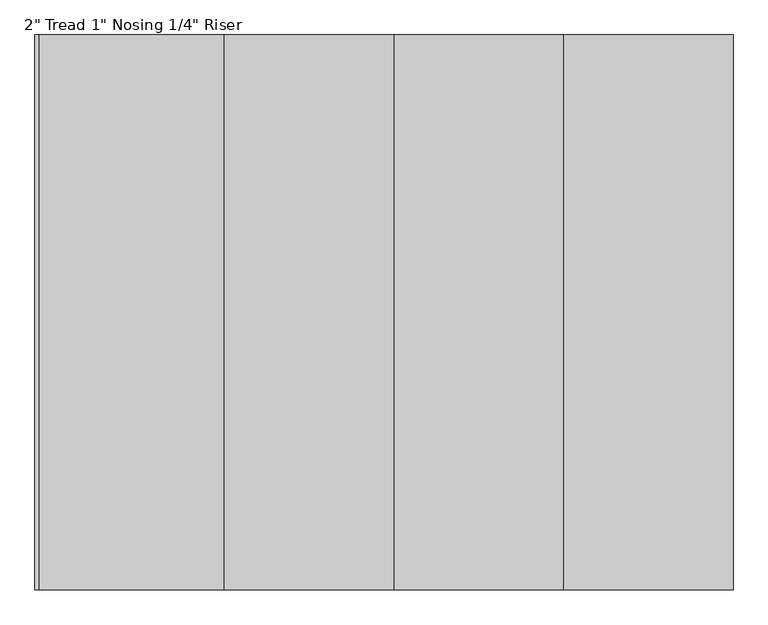
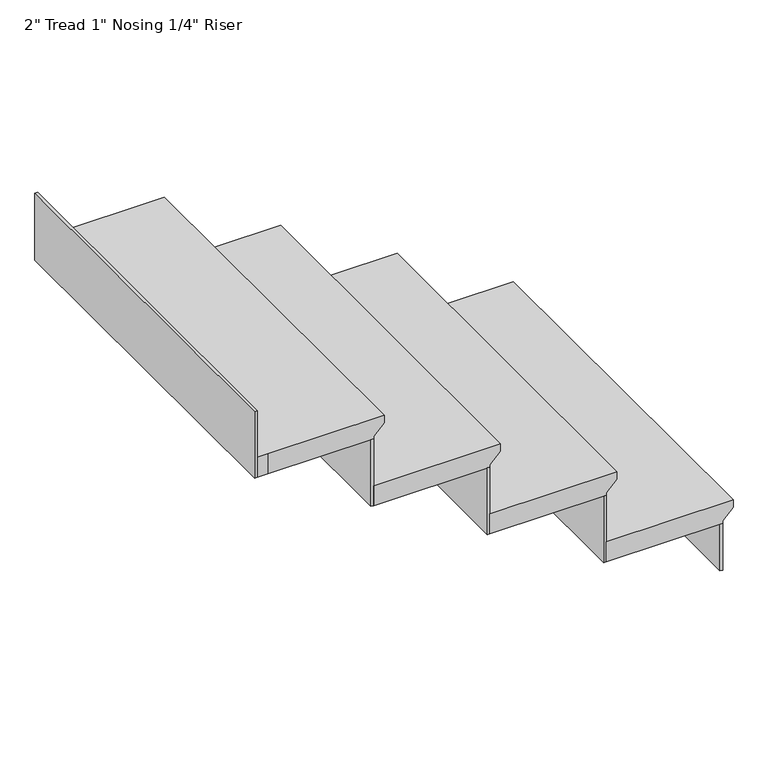
"""IFC4 building model written with IfcOpenShell, lengths in millimetres: stair flight geometry."""

from ifc_helpers import new_model, si_unit, origin, place, context, project, spatial, faceted_brep, source, transform, mapped, element, save


def stair_flight_f80b6bc8(model_context):
    return source(origin(), model_context, "Body", "Brep", [
        faceted_brep([(-9079.7156858, 1045.1115003, 3503.0833333), (-9079.7156858, 1045.1115003, 3522.1333333), (-9079.7156858, 130.7115003, 3522.1333333), (-9079.7156858, 130.7115003, 3503.0833333), (-9105.1156858, 1045.1115003, 3477.6833333), (-9105.1156858, 130.7115003, 3477.6833333), (-9384.5156858, 1045.1115003, 3522.1333333), (-9384.5156858, 130.7115003, 3522.1333333), (-9105.1156858, 130.7115003, 3471.3333333), (-9384.5156858, 130.7115003, 3471.3333333), (-9384.5156858, 1045.1115003, 3471.3333333), (-9105.1156858, 1045.1115003, 3471.3333333)], [[[0, 1, 2, 3]], [[4, 0, 3, 5]], [[2, 1, 6, 7]], [[8, 9, 10, 11]], [[2, 7, 9, 8, 5, 3]], [[8, 11, 4, 5]], [[6, 1, 0, 4, 11, 10]], [[7, 6, 10, 9]]]),
        faceted_brep([(-9105.1156858, 1045.1115003, 3471.3333333), (-9105.1156858, 1045.1115003, 3352.8), (-9111.4656858, 1045.1115003, 3352.8), (-9111.4656858, 1045.1115003, 3471.3333333), (-9105.1156858, 130.7115003, 3471.3333333), (-9111.4656858, 130.7115003, 3471.3333333), (-9111.4656858, 130.7115003, 3352.8), (-9105.1156858, 130.7115003, 3352.8)], [[[0, 1, 2, 3]], [[4, 5, 6, 7]], [[1, 0, 4, 7]], [[2, 1, 7, 6]], [[3, 2, 6, 5]], [[0, 3, 5, 4]]]),
        faceted_brep([(-9384.5156858, 1045.1115003, 3640.6666667), (-9384.5156858, 1045.1115003, 3471.3333333), (-9390.8656858, 1045.1115003, 3471.3333333), (-9390.8656858, 1045.1115003, 3640.6666667), (-9384.5156858, 130.7115003, 3640.6666667), (-9390.8656858, 130.7115003, 3640.6666667), (-9390.8656858, 130.7115003, 3471.3333333), (-9384.5156858, 130.7115003, 3471.3333333)], [[[0, 1, 2, 3]], [[4, 5, 6, 7]], [[1, 0, 4, 7]], [[2, 1, 7, 6]], [[3, 2, 6, 5]], [[0, 3, 5, 4]]]),
        faceted_brep([(-9359.1156858, 130.7115003, 3691.4666667), (-9359.1156858, 1045.1115003, 3691.4666667), (-9663.9156858, 1045.1115003, 3691.4666667), (-9663.9156858, 130.7115003, 3691.4666667), (-9384.5156858, 130.7115003, 3640.6666667), (-9663.9156858, 130.7115003, 3640.6666667), (-9663.9156858, 1045.1115003, 3640.6666667), (-9384.5156858, 1045.1115003, 3640.6666667), (-9384.5156858, 130.7115003, 3647.0166667), (-9359.1156858, 130.7115003, 3672.4166667), (-9384.5156858, 1045.1115003, 3647.0166667), (-9359.1156858, 1045.1115003, 3672.4166667)], [[[0, 1, 2, 3]], [[4, 5, 6, 7]], [[0, 3, 5, 4, 8, 9]], [[4, 7, 10, 8]], [[2, 1, 11, 10, 7, 6]], [[3, 2, 6, 5]], [[11, 1, 0, 9]], [[10, 11, 9, 8]]]),
        faceted_brep([(-9663.9156858, 1045.1115003, 3810.0), (-9663.9156858, 1045.1115003, 3640.6666667), (-9670.2656858, 1045.1115003, 3640.6666667), (-9670.2656858, 1045.1115003, 3810.0), (-9663.9156858, 130.7115003, 3810.0), (-9670.2656858, 130.7115003, 3810.0), (-9670.2656858, 130.7115003, 3640.6666667), (-9663.9156858, 130.7115003, 3640.6666667)], [[[0, 1, 2, 3]], [[4, 5, 6, 7]], [[1, 0, 4, 7]], [[2, 1, 7, 6]], [[3, 2, 6, 5]], [[0, 3, 5, 4]]]),
        faceted_brep([(-9638.5156858, 130.7115003, 3860.8), (-9638.5156858, 1045.1115003, 3860.8), (-9943.3156858, 1045.1115003, 3860.8), (-9943.3156858, 130.7115003, 3860.8), (-9663.9156858, 130.7115003, 3810.0), (-9943.3156858, 130.7115003, 3810.0), (-9943.3156858, 1045.1115003, 3810.0), (-9663.9156858, 1045.1115003, 3810.0), (-9663.9156858, 130.7115003, 3816.35), (-9638.5156858, 130.7115003, 3841.75), (-9663.9156858, 1045.1115003, 3816.35), (-9638.5156858, 1045.1115003, 3841.75)], [[[0, 1, 2, 3]], [[4, 5, 6, 7]], [[0, 3, 5, 4, 8, 9]], [[4, 7, 10, 8]], [[2, 1, 11, 10, 7, 6]], [[3, 2, 6, 5]], [[11, 1, 0, 9]], [[10, 11, 9, 8]]]),
        faceted_brep([(-10222.7156858, 1045.1115003, 4148.6666667), (-10222.7156858, 1045.1115003, 3979.3333333), (-10229.0656858, 1045.1115003, 3979.3333333), (-10229.0656858, 1045.1115003, 4148.6666667), (-10222.7156858, 130.7115003, 4148.6666667), (-10229.0656858, 130.7115003, 4148.6666667), (-10229.0656858, 130.7115003, 3979.3333333), (-10222.7156858, 130.7115003, 3979.3333333)], [[[0, 1, 2, 3]], [[4, 5, 6, 7]], [[1, 0, 4, 7]], [[2, 1, 7, 6]], [[3, 2, 6, 5]], [[0, 3, 5, 4]]]),
        faceted_brep([(-9943.3156858, 1045.1115003, 3979.3333333), (-9943.3156858, 1045.1115003, 3810.0), (-9949.6656858, 1045.1115003, 3810.0), (-9949.6656858, 1045.1115003, 3979.3333333), (-9943.3156858, 130.7115003, 3979.3333333), (-9949.6656858, 130.7115003, 3979.3333333), (-9949.6656858, 130.7115003, 3810.0), (-9943.3156858, 130.7115003, 3810.0)], [[[0, 1, 2, 3]], [[4, 5, 6, 7]], [[1, 0, 4, 7]], [[2, 1, 7, 6]], [[3, 2, 6, 5]], [[0, 3, 5, 4]]]),
        faceted_brep([(-10222.7156858, 130.7115003, 4030.1333333), (-10197.3156858, 130.7115003, 4030.1333333), (-9917.9156858, 130.7115003, 4030.1333333), (-9917.9156858, 1045.1115003, 4030.1333333), (-10197.3156858, 1045.1115003, 4030.1333333), (-10222.7156858, 1045.1115003, 4030.1333333), (-10197.3156858, 130.7115003, 3979.3333333), (-10222.7156858, 130.7115003, 3979.3333333), (-10222.7156858, 1045.1115003, 3979.3333333), (-10197.3156858, 1045.1115003, 3979.3333333), (-9943.3156858, 1045.1115003, 3979.3333333), (-9943.3156858, 130.7115003, 3979.3333333), (-9943.3156858, 130.7115003, 3985.6833333), (-9917.9156858, 130.7115003, 4011.0833333), (-9943.3156858, 1045.1115003, 3985.6833333), (-9917.9156858, 1045.1115003, 4011.0833333)], [[[0, 1, 2, 3, 4, 5]], [[6, 7, 8, 9, 10, 11]], [[1, 0, 7, 6]], [[2, 1, 6, 11, 12, 13]], [[11, 10, 14, 12]], [[4, 3, 15, 14, 10, 9]], [[5, 4, 9, 8]], [[0, 5, 8, 7]], [[15, 3, 2, 13]], [[14, 15, 13, 12]]]),
    ])


if __name__ == "__main__":
    model = new_model("IFC4")
    model_context = context("Model", 3, world=origin())
    ifc_project = project(units=[si_unit("LENGTHUNIT", "METRE", prefix="MILLI")], contexts=[model_context])
    site = spatial("IfcSite", under=ifc_project)
    building = spatial("IfcBuilding", under=site)
    placement = place(None, origin())
    stair_flight_shape = stair_flight_f80b6bc8(model_context)
    element("IfcStairFlight", 1, ObjectType="2\" Tread 1\" Nosing 1/4\" Riser", at=placement, inside=building, context=model_context, shape_type="MappedRepresentation", body=[
        mapped(stair_flight_shape, transform((0.0, 0.0, 0.0), x_axis=(1.0, 0.0, 0.0), y_axis=(0.0, 1.0, 0.0), z_axis=(0.0, 0.0, 1.0))),
    ])
    save(model, "model.ifc")
